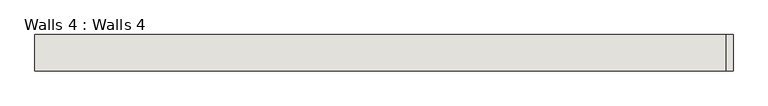
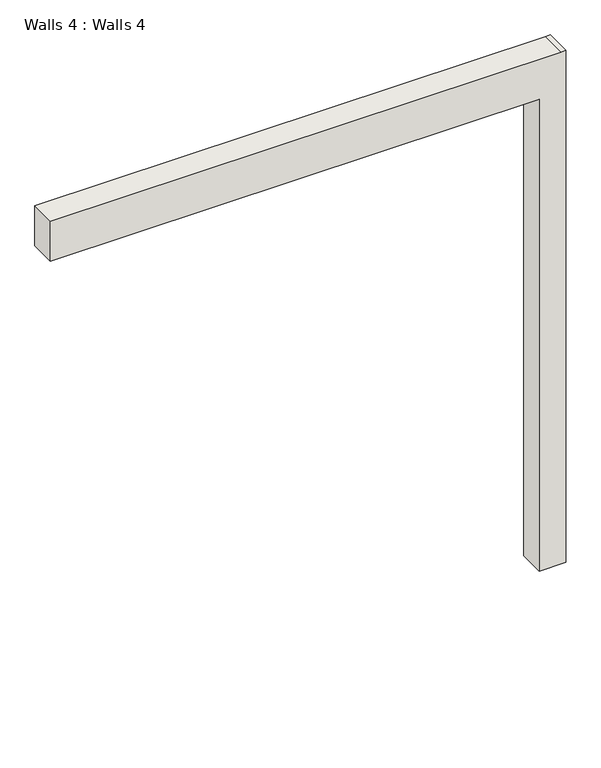
"""IFC4 building model written with IfcOpenShell, lengths in millimetres: wall geometry, Walls 4 : Walls 4."""

from ifc_helpers import new_model, si_unit, frame, origin, place, context, project, spatial, polyline, outline, extrude, source, transform, mapped, element, save


def walls_4_walls_4_3dff52d5(model_context):
    return source(origin(), model_context, "Body", "SweptSolid", [
        extrude(outline(polyline([(6148.0, 13234.1864069), (6148.0, 7439.6639497), (5665.4, 7439.6639497), (5665.4, 12989.0008502), (0.0, 12989.0008502), (0.0, 13293.8008502), (6148.0, 13293.8008502), (6148.0, 13234.1864069)])), frame((0.0, -266.6843256, 0.0), z_axis=(0.0, 1.0, 0.0), x_axis=(0.0, 0.0, 1.0)), (0.0, 0.0, 1.0), 304.8),
    ])


if __name__ == "__main__":
    model = new_model("IFC4")
    model_context = context("Model", 3, world=origin())
    ifc_project = project(units=[si_unit("LENGTHUNIT", "METRE", prefix="MILLI")], contexts=[model_context])
    site = spatial("IfcSite", under=ifc_project)
    building = spatial("IfcBuilding", under=site)
    placement = place(None, origin())
    walls_4_walls_4_shape = walls_4_walls_4_3dff52d5(model_context)
    element("IfcWall", 1, ObjectType="Walls 4 : Walls 4", at=placement, inside=building, context=model_context, shape_type="MappedRepresentation", body=[
        mapped(walls_4_walls_4_shape, transform((0.0, 0.0, 0.0), x_axis=(1.0, 0.0, 0.0), y_axis=(0.0, 1.0, 0.0), z_axis=(0.0, 0.0, 1.0))),
    ])
    save(model, "model.ifc")

# Revit data of these elements
# Element 1 (IfcWall, "Walls 4 : Walls 4")
#   Materials on its faces: "Default Wall"
# Materials
#   "Default Wall": colour RGB 80 80 80, transparency 0
